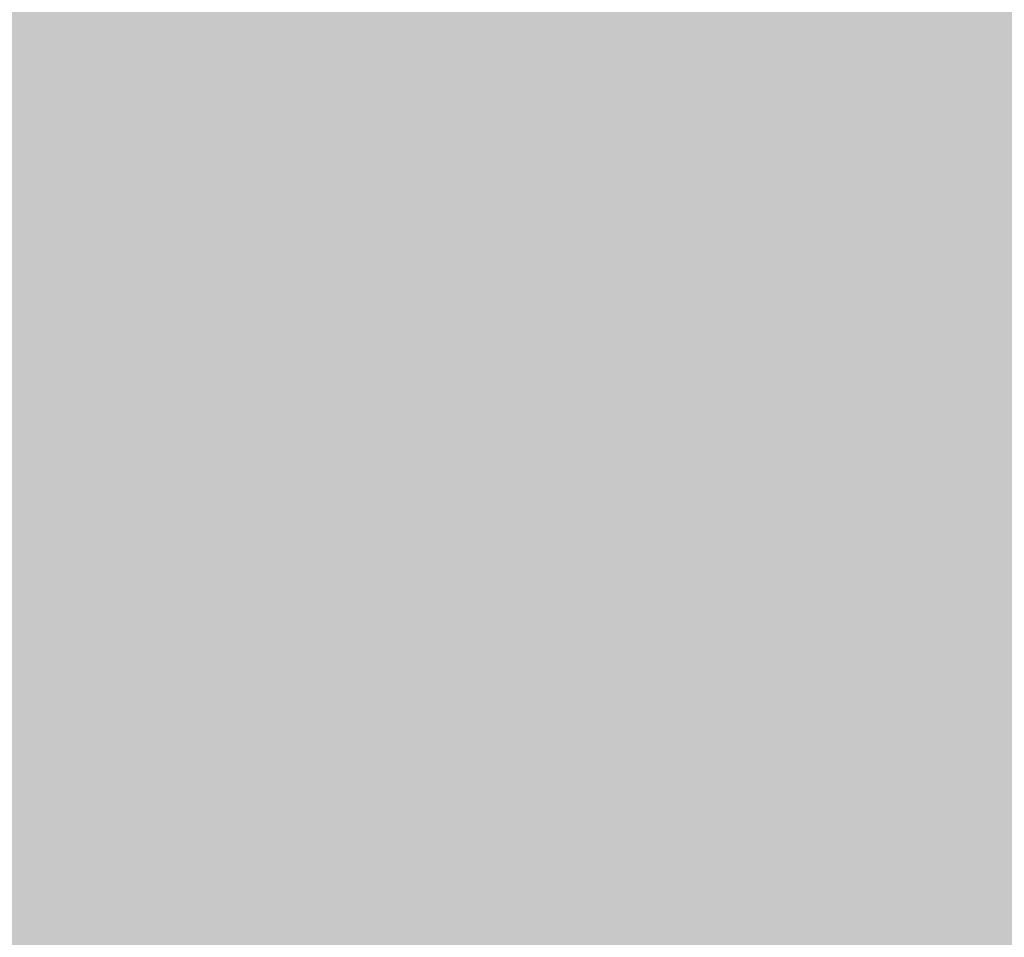
# Model space of a CAD drawing. Units: millimetres. Extents: x 0 to 2267, y 0 to 1823.
# Tile 143 of 256: x 1802 to 1823, y 1132 to 1152. Entities that reach past the tile are written whole.
import ezdxf

# ---------------------------------------------------------------- set-up
doc = ezdxf.new("R2010")
doc.units = ezdxf.units.MM
doc.header["$MEASUREMENT"] = 0
doc.layers.add('M-HATC', color=252, linetype='Continuous', lineweight=18)

msp = doc.modelspace()

# ---------------------------------------------------------------- hatches: boundary and pattern name
at = {"layer": 'M-HATC'}
h = msp.add_hatch(color=256, dxfattribs=at)
h.dxf.hatch_style = 1
h.paths.add_polyline_path([(2055.771, 1603.062), (1381.087, 1603.062), (1381.087, 1598.062), (2055.771, 1598.062)])
h.paths.add_polyline_path([(2055.771, 1598.062), (1381.087, 1598.062), (1381.087, 1593.062), (2055.771, 1593.062)])
h.paths.add_polyline_path([(2051.307, 1536.761), (1385.55, 1536.761), (1385.55, 1526.761), (1387.55, 1526.761), (1388.537, 1525.053), (1385.332, 1521.233), (1385.332, 1521.223), (2050.254, 1522.749), (2048.321, 1525.053), (2049.307, 1526.761), (2051.307, 1526.761)])
edge = h.paths.add_edge_path()
edge.add_arc((1847.535, 1379.149), 135, 222.60306, 222.89085, ccw=False)
edge.add_line((1748.166, 1287.766), (1683.092, 1287.766))
edge.add_arc((1583.724, 1379.149), 135, 317.10915, 317.39694, ccw=False)
edge.add_arc((1678.969, 1290.671), 5, 222.8909, 317.1091, ccw=False)
edge.add_arc((1774.213, 1379.149), 135, 222.60306, 222.89085, ccw=False)
edge.add_line((1674.845, 1287.766), (1609.771, 1287.766))
edge.add_arc((1510.403, 1379.149), 135, 317.10915, 317.39694, ccw=False)
edge.add_arc((1605.647, 1290.671), 5, 222.8909, 317.1091, ccw=False)
edge.add_arc((1700.892, 1379.149), 135, 222.60306, 222.89085, ccw=False)
edge.add_line((1601.524, 1287.766), (1536.45, 1287.766))
edge.add_arc((1437.081, 1379.149), 135, 317.10915, 317.39694, ccw=False)
edge.add_arc((1532.326, 1290.671), 5, 222.8909, 317.1091, ccw=False)
edge.add_arc((1627.571, 1379.149), 135, 222.60306, 222.89085, ccw=False)
edge.add_line((1528.203, 1287.766), (1505.929, 1287.766))
edge.add_spline(control_points=[(1505.929, 1287.766), (1504.262, 1287.766), (1504.262, 1282.766), (1505.929, 1282.766)], knot_values=[0, 0, 0, 0, 5, 5, 5, 5], degree=3, periodic=0)
edge.add_line((1505.929, 1282.766), (1930.929, 1282.766))
edge.add_spline(control_points=[(1930.929, 1282.766), (1932.596, 1282.766), (1932.596, 1287.766), (1930.929, 1287.766)], knot_values=[0, 0, 0, 0, 5, 5, 5, 5], degree=3, periodic=0)
edge.add_line((1930.929, 1287.766), (1903.056, 1287.766))
edge.add_arc((1803.688, 1379.149), 135, 317.10915, 317.39694, ccw=False)
edge.add_arc((1898.932, 1290.671), 5, 222.8909, 317.1091, ccw=False)
edge.add_arc((1994.177, 1379.149), 135, 222.60306, 222.89085, ccw=False)
edge.add_line((1894.809, 1287.766), (1829.735, 1287.766))
edge.add_arc((1730.366, 1379.149), 135, 317.10915, 317.39694, ccw=False)
edge.add_arc((1825.611, 1290.671), 5, 222.8909, 317.1091, ccw=False)
edge.add_arc((1920.856, 1379.149), 135, 222.60306, 222.89085, ccw=False)
edge.add_line((1821.487, 1287.766), (1756.413, 1287.766))
edge.add_arc((1657.045, 1379.149), 135, 317.10915, 317.39694, ccw=False)
edge.add_arc((1752.29, 1290.671), 5, 222.8909, 317.1091, ccw=False)
edge = h.paths.add_edge_path()
edge.add_spline(control_points=[(1843.429, 1227.247), (1845.096, 1227.247), (1845.096, 1232.247), (1843.429, 1232.247)], knot_values=[0, 0, 0, 0, 5, 5, 5, 5], degree=3, periodic=0)
edge.add_line((1843.429, 1232.247), (1593.429, 1232.247))
edge.add_spline(control_points=[(1593.429, 1232.247), (1591.762, 1232.247), (1591.762, 1227.247), (1593.429, 1227.247)], knot_values=[0, 0, 0, 0, 5, 5, 5, 5], degree=3, periodic=0)
edge.add_line((1593.429, 1227.247), (1843.429, 1227.247))
h.paths.add_polyline_path([(1905.929, 1127.417), (1530.929, 1127.417, 0.414214), (1520.929, 1117.417), (1530.929, 1117.417), (1915.929, 1117.417, 0.414214)])
edge = h.paths.add_edge_path()
edge.add_arc((1397.086, 1498.408), 12.73, 90.7821, 190.8787, ccw=False)
edge.add_line((1396.912, 1511.136), (1428.01, 1511.349))
edge.add_line((1428.01, 1511.349), (1433.01, 1511.349))
edge.add_line((1433.01, 1511.349), (1434.439, 1511.349))
edge.add_arc((1419.474, 1498.08), 20, 41.561, 74.0821)
edge.add_line((1424.959, 1517.314), (1399.935, 1517.256))
edge.add_spline(control_points=[(1399.931, 1517.256), (1399.884, 1517.213), (1399.833, 1517.169), (1399.777, 1517.124)], knot_values=[11.567499, 11.567499, 11.567499, 11.567499, 11.814249, 11.814249, 11.814249, 11.814249], degree=3, periodic=0)
edge.add_spline(control_points=[(1399.633, 1517.01), (1399.583, 1516.972), (1399.531, 1516.934), (1399.476, 1516.895)], knot_values=[11.167718, 11.167718, 11.167718, 11.167718, 11.365188, 11.365188, 11.365188, 11.365188], degree=3, periodic=0)
edge.add_spline(control_points=[(1399.34, 1516.8), (1399.151, 1516.672), (1398.938, 1516.538), (1398.704, 1516.399)], knot_values=[10.376405, 10.376405, 10.376405, 10.376405, 11.00994, 11.00994, 11.00994, 11.00994], degree=3, periodic=0)
edge.add_spline(control_points=[(1398.657, 1516.372), (1398.579, 1516.326), (1398.498, 1516.28), (1398.415, 1516.233)], knot_values=[10.125175, 10.125175, 10.125175, 10.125175, 10.334406, 10.334406, 10.334406, 10.334406], degree=3, periodic=0)
edge.add_spline(control_points=[(1398.264, 1516.149), (1398.196, 1516.111), (1398.126, 1516.073), (1398.055, 1516.035)], knot_values=[9.832246, 9.832246, 9.832246, 9.832246, 9.999658, 9.999658, 9.999658, 9.999658], degree=3, periodic=0)
edge.add_spline(control_points=[(1397.999, 1516.005), (1397.731, 1515.862), (1397.446, 1515.717), (1397.147, 1515.571)], knot_values=[9.161808, 9.161808, 9.161808, 9.161808, 9.787769, 9.787769, 9.787769, 9.787769], degree=3, periodic=0)
edge.add_spline(control_points=[(1397.147, 1515.571), (1396.842, 1515.423), (1396.522, 1515.274), (1396.191, 1515.126)], knot_values=[8.524455, 8.524455, 8.524455, 8.524455, 9.161808, 9.161808, 9.161808, 9.161808], degree=3, periodic=0)
edge.add_spline(control_points=[(1396.078, 1515.076), (1395.985, 1515.035), (1395.892, 1514.994), (1395.798, 1514.953)], knot_values=[8.275193, 8.275193, 8.275193, 8.275193, 8.451726, 8.451726, 8.451726, 8.451726], degree=3, periodic=0)
edge.add_spline(control_points=[(1395.602, 1514.869), (1395.5, 1514.826), (1395.397, 1514.782), (1395.293, 1514.739)], knot_values=[7.962917, 7.962917, 7.962917, 7.962917, 8.152764, 8.152764, 8.152764, 8.152764], degree=3, periodic=0)
edge.add_spline(control_points=[(1395.212, 1514.706), (1394.828, 1514.547), (1394.435, 1514.393), (1394.036, 1514.244)], knot_values=[7.21254, 7.21254, 7.21254, 7.21254, 7.913148, 7.913148, 7.913148, 7.913148], degree=3, periodic=0)
edge.add_spline(control_points=[(1394.036, 1514.244), (1393.708, 1514.121), (1393.375, 1514.003), (1393.043, 1513.889)], knot_values=[6.633733, 6.633733, 6.633733, 6.633733, 7.21254, 7.21254, 7.21254, 7.21254], degree=3, periodic=0)
edge.add_spline(control_points=[(1392.821, 1513.815), (1392.72, 1513.781), (1392.618, 1513.748), (1392.517, 1513.715)], knot_values=[6.328796, 6.328796, 6.328796, 6.328796, 6.505493, 6.505493, 6.505493, 6.505493], degree=3, periodic=0)
edge.add_spline(control_points=[(1392.517, 1513.715), (1392.319, 1513.652), (1392.121, 1513.59), (1391.924, 1513.531)], knot_values=[5.984605, 5.984605, 5.984605, 5.984605, 6.328796, 6.328796, 6.328796, 6.328796], degree=3, periodic=0)
edge.add_spline(control_points=[(1391.792, 1513.491), (1391.312, 1513.35), (1390.838, 1513.224), (1390.378, 1513.117)], knot_values=[5.066697, 5.066697, 5.066697, 5.066697, 5.907055, 5.907055, 5.907055, 5.907055], degree=3, periodic=0)
edge.add_spline(control_points=[(1390.378, 1513.117), (1390.18, 1513.071), (1389.984, 1513.028), (1389.791, 1512.99)], knot_values=[4.70367, 4.70367, 4.70367, 4.70367, 5.066695, 5.066695, 5.066695, 5.066695], degree=3, periodic=0)
edge.add_spline(control_points=[(1389.422, 1512.92), (1389.246, 1512.889), (1389.073, 1512.862), (1388.904, 1512.838)], knot_values=[4.130571, 4.130571, 4.130571, 4.130571, 4.469816, 4.469816, 4.469816, 4.469816], degree=3, periodic=0)
edge.add_spline(control_points=[(1388.904, 1512.838), (1388.591, 1512.795), (1388.291, 1512.764), (1388.007, 1512.749)], knot_values=[3.504031, 3.504031, 3.504031, 3.504031, 4.130571, 4.130571, 4.130571, 4.130571], degree=3, periodic=0)
edge.add_spline(control_points=[(1387.936, 1512.746), (1387.854, 1512.742), (1387.773, 1512.74), (1387.694, 1512.739)], knot_values=[3.268866, 3.268866, 3.268866, 3.268866, 3.451164, 3.451164, 3.451164, 3.451164], degree=3, periodic=0)
edge.add_spline(control_points=[(1387.335, 1512.744), (1387.208, 1512.75), (1387.085, 1512.76), (1386.967, 1512.774)], knot_values=[2.670686, 2.670686, 2.670686, 2.670686, 2.984, 2.984, 2.984, 2.984], degree=3, periodic=0)
edge.add_spline(control_points=[(1386.833, 1512.792), (1386.821, 1512.794), (1386.809, 1512.796), (1386.797, 1512.798)], knot_values=[2.516981, 2.516981, 2.516981, 2.516981, 2.549528, 2.549528, 2.549528, 2.549528], degree=3, periodic=0)
edge.add_spline(control_points=[(1386.453, 1512.873), (1386.426, 1512.881), (1386.399, 1512.889), (1386.373, 1512.897)], knot_values=[2.095869, 2.095869, 2.095869, 2.095869, 2.17941, 2.17941, 2.17941, 2.17941], degree=3, periodic=0)
edge.add_spline(control_points=[(1386.069, 1513.019), (1386.063, 1513.022), (1386.058, 1513.025), (1386.052, 1513.028)], knot_values=[1.72453, 1.72453, 1.72453, 1.72453, 1.745933, 1.745933, 1.745933, 1.745933], degree=3, periodic=0)
edge.add_arc((1399.474, 1498.08), 20, 131.8243, 180)
edge.add_arc((1630.334, 1505.548), 250.971, 181.70518, 236.42798)
edge.add_arc((1605.34, 1483.304), 218.782, 238.66083, 243.34961)
edge.add_arc((1647.091, 1510.359), 262.899, 183.12984, 237.85344, ccw=False)
h.paths.add_polyline_path([(1406.537, 1391.964, 0.149382), (1491.551, 1296.442, -0.129517)], flags=17)
edge = h.paths.add_edge_path()
edge.add_arc((2037.384, 1498.08), 20, 0, 48.2659)
edge.add_spline(control_points=[(2050.697, 1513.005), (2050.651, 1512.985), (2050.603, 1512.966), (2050.554, 1512.948)], knot_values=[1.835652, 1.835652, 1.835652, 1.835652, 2.000781, 2.000781, 2.000781, 2.000781], degree=3, periodic=0)
edge.add_spline(control_points=[(2050.462, 1512.917), (2050.479, 1512.922), (2050.496, 1512.928), (2050.513, 1512.934)], knot_values=[2.045477, 2.045477, 2.045477, 2.045477, 2.101389, 2.101389, 2.101389, 2.101389], degree=3, periodic=0)
edge.add_spline(control_points=[(2050.129, 1512.834), (2050.198, 1512.847), (2050.266, 1512.862), (2050.331, 1512.879)], knot_values=[2.237629, 2.237629, 2.237629, 2.237629, 2.435841, 2.435841, 2.435841, 2.435841], degree=3, periodic=0)
edge.add_spline(control_points=[(2050.095, 1512.828), (2050.106, 1512.83), (2050.118, 1512.832), (2050.129, 1512.834)], knot_values=[2.435841, 2.435841, 2.435841, 2.435841, 2.468321, 2.468321, 2.468321, 2.468321], degree=3, periodic=0)
edge.add_spline(control_points=[(2049.784, 1512.785), (2049.855, 1512.792), (2049.924, 1512.801), (2049.992, 1512.811)], knot_values=[2.563852, 2.563852, 2.563852, 2.563852, 2.748541, 2.748541, 2.748541, 2.748541], degree=3, periodic=0)
edge.add_spline(control_points=[(2049.405, 1512.762), (2049.536, 1512.765), (2049.663, 1512.773), (2049.784, 1512.785)], knot_values=[2.748541, 2.748541, 2.748541, 2.748541, 3.064882, 3.064882, 3.064882, 3.064882], degree=3, periodic=0)
edge.add_spline(control_points=[(2049.17, 1512.76), (2049.234, 1512.759), (2049.297, 1512.759), (2049.358, 1512.761)], knot_values=[3.102309, 3.102309, 3.102309, 3.102309, 3.2503, 3.2503, 3.2503, 3.2503], degree=3, periodic=0)
edge.add_spline(control_points=[(2048.857, 1512.769), (2048.964, 1512.764), (2049.068, 1512.761), (2049.17, 1512.76)], knot_values=[3.2503, 3.2503, 3.2503, 3.2503, 3.486069, 3.486069, 3.486069, 3.486069], degree=3, periodic=0)
edge.add_spline(control_points=[(2048.692, 1512.779), (2048.373, 1512.801), (2048.035, 1512.841), (2047.682, 1512.897)], knot_values=[3.606429, 3.606429, 3.606429, 3.606429, 4.2989, 4.2989, 4.2989, 4.2989], degree=3, periodic=0)
edge.add_spline(control_points=[(2047.682, 1512.897), (2047.546, 1512.919), (2047.408, 1512.942), (2047.268, 1512.969)], knot_values=[4.2989, 4.2989, 4.2989, 4.2989, 4.565769, 4.565769, 4.565769, 4.565769], degree=3, periodic=0)
edge.add_spline(control_points=[(2047.268, 1512.969), (2047.145, 1512.991), (2047.021, 1513.016), (2046.895, 1513.042)], knot_values=[4.565769, 4.565769, 4.565769, 4.565769, 4.799971, 4.799971, 4.799971, 4.799971], degree=3, periodic=0)
edge.add_spline(control_points=[(2046.895, 1513.042), (2046.529, 1513.119), (2046.151, 1513.209), (2045.768, 1513.311)], knot_values=[4.799971, 4.799971, 4.799971, 4.799971, 5.483718, 5.483718, 5.483718, 5.483718], degree=3, periodic=0)
edge.add_spline(control_points=[(2045.768, 1513.311), (2045.372, 1513.415), (2044.97, 1513.532), (2044.566, 1513.659)], knot_values=[5.483718, 5.483718, 5.483718, 5.483718, 6.187866, 6.187866, 6.187866, 6.187866], degree=3, periodic=0)
edge.add_spline(control_points=[(2044.566, 1513.659), (2044.415, 1513.706), (2044.263, 1513.755), (2044.112, 1513.805)], knot_values=[6.187866, 6.187866, 6.187866, 6.187866, 6.451551, 6.451551, 6.451551, 6.451551], degree=3, periodic=0)
edge.add_spline(control_points=[(2044.112, 1513.805), (2043.997, 1513.843), (2043.882, 1513.881), (2043.767, 1513.92)], knot_values=[6.451551, 6.451551, 6.451551, 6.451551, 6.651434, 6.651434, 6.651434, 6.651434], degree=3, periodic=0)
edge.add_spline(control_points=[(2043.767, 1513.92), (2043.372, 1514.055), (2042.977, 1514.198), (2042.589, 1514.346)], knot_values=[6.651434, 6.651434, 6.651434, 6.651434, 7.338879, 7.338879, 7.338879, 7.338879], degree=3, periodic=0)
edge.add_spline(control_points=[(2042.589, 1514.346), (2042.164, 1514.507), (2041.746, 1514.675), (2041.341, 1514.846)], knot_values=[7.338879, 7.338879, 7.338879, 7.338879, 8.089209, 8.089209, 8.089209, 8.089209], degree=3, periodic=0)
edge.add_spline(control_points=[(2041.341, 1514.846), (2041.103, 1514.946), (2040.869, 1515.048), (2040.64, 1515.15)], knot_values=[8.089209, 8.089209, 8.089209, 8.089209, 8.529587, 8.529587, 8.529587, 8.529587], degree=3, periodic=0)
edge.add_spline(control_points=[(2040.51, 1515.209), (2040.082, 1515.402), (2039.675, 1515.597), (2039.295, 1515.789)], knot_values=[8.613818, 8.613818, 8.613818, 8.613818, 9.44571, 9.44571, 9.44571, 9.44571], degree=3, periodic=0)
edge.add_spline(control_points=[(2039.295, 1515.789), (2039.062, 1515.907), (2038.839, 1516.025), (2038.629, 1516.14)], knot_values=[9.44571, 9.44571, 9.44571, 9.44571, 9.956404, 9.956404, 9.956404, 9.956404], degree=3, periodic=0)
edge.add_spline(control_points=[(2038.629, 1516.14), (2038.519, 1516.2), (2038.412, 1516.26), (2038.309, 1516.319)], knot_values=[9.956404, 9.956404, 9.956404, 9.956404, 10.223542, 10.223542, 10.223542, 10.223542], degree=3, periodic=0)
edge.add_spline(control_points=[(2038.309, 1516.319), (2038.214, 1516.374), (2038.122, 1516.428), (2038.033, 1516.481)], knot_values=[10.223542, 10.223542, 10.223542, 10.223542, 10.47051, 10.47051, 10.47051, 10.47051], degree=3, periodic=0)
edge.add_spline(control_points=[(2038.033, 1516.481), (2037.786, 1516.63), (2037.564, 1516.773), (2037.372, 1516.909)], knot_values=[10.47051, 10.47051, 10.47051, 10.47051, 11.15767, 11.15767, 11.15767, 11.15767], degree=3, periodic=0)
edge.add_spline(control_points=[(2037.372, 1516.909), (2037.279, 1516.975), (2037.193, 1517.04), (2037.114, 1517.102)], knot_values=[11.15767, 11.15767, 11.15767, 11.15767, 11.49227, 11.49227, 11.49227, 11.49227], degree=3, periodic=0)
edge.add_spline(control_points=[(2036.856, 1517.326), (2036.915, 1517.269), (2036.981, 1517.21), (2037.056, 1517.149)], knot_values=[11.577341, 11.577341, 11.577341, 11.577341, 11.91035, 11.91035, 11.91035, 11.91035], degree=3, periodic=0)
edge.add_spline(control_points=[(2036.807, 1517.375), (2036.823, 1517.359), (2036.839, 1517.342), (2036.856, 1517.326)], knot_values=[11.91035, 11.91035, 11.91035, 11.91035, 12.007402, 12.007402, 12.007402, 12.007402], degree=3, periodic=0)
edge.add_spline(control_points=[(2036.702, 1517.494), (2036.71, 1517.483), (2036.72, 1517.472), (2036.729, 1517.461)], knot_values=[12.184155, 12.184155, 12.184155, 12.184155, 12.255409, 12.255409, 12.255409, 12.255409], degree=3, periodic=0)
edge.add_spline(control_points=[(2036.616, 1517.621), (2036.62, 1517.613), (2036.624, 1517.606), (2036.629, 1517.598)], knot_values=[12.487913, 12.487913, 12.487913, 12.487913, 12.541035, 12.541035, 12.541035, 12.541035], degree=3, periodic=0)
edge.add_spline(control_points=[(2036.563, 1517.786), (2036.564, 1517.779), (2036.564, 1517.773), (2036.565, 1517.766)], knot_values=[12.911761, 12.911761, 12.911761, 12.911761, 12.968286, 12.968286, 12.968286, 12.968286], degree=3, periodic=0)
edge.add_spline(control_points=[(2036.617, 1517.93), (2036.612, 1517.926), (2036.609, 1517.921), (2036.605, 1517.916)], knot_values=[13.382527, 13.382527, 13.382527, 13.382527, 13.433791, 13.433791, 13.433791, 13.433791], degree=3, periodic=0)
edge.add_spline(control_points=[(2036.749, 1518.017), (2036.736, 1518.012), (2036.724, 1518.006), (2036.712, 1518)], knot_values=[13.726299, 13.726299, 13.726299, 13.726299, 13.809928, 13.809928, 13.809928, 13.809928], degree=3, periodic=0)
edge.add_spline(control_points=[(2036.86, 1518.053), (2036.839, 1518.047), (2036.818, 1518.042), (2036.799, 1518.035)], knot_values=[13.910887, 13.910887, 13.910887, 13.910887, 14.02153, 14.02153, 14.02153, 14.02153], degree=3, periodic=0)
edge.add_line((2036.964, 1518.08), (2032.384, 1518.08))
edge.add_line((2032.384, 1518.08), (2027.384, 1518.08))
edge.add_line((2027.384, 1518.08), (2022.384, 1518.08))
edge.add_line((2022.384, 1518.08), (2017.384, 1518.08))
edge.add_arc((2017.384, 1498.08), 20, 90, 138.439)
edge.add_line((2002.419, 1511.349), (2003.848, 1511.349))
edge.add_line((2003.848, 1511.349), (2008.848, 1511.349))
edge.add_line((2008.848, 1511.349), (2039.772, 1511.138))
edge.add_arc((2039.772, 1498.408), 12.73, -10.8787, 90, ccw=False)
edge.add_arc((1789.767, 1510.359), 262.899, 302.14656, 356.87016, ccw=False)
edge.add_arc((1831.518, 1483.304), 218.782, 296.65039, 301.33917)
edge.add_arc((1806.524, 1505.548), 250.971, 303.57202, 358.29482)
h.paths.add_polyline_path([(2030.321, 1391.964, -0.129517), (1945.307, 1296.442, 0.149382)], flags=17)
edge = h.paths.add_edge_path()
edge.add_spline(control_points=[(2037.246, 1518.082), (2037.29, 1518.081), (2037.336, 1518.08), (2037.384, 1518.08)], knot_values=[0.000012, 0.000012, 0.000012, 0.000012, 0.144754, 0.144754, 0.144754, 0.144754], degree=3, periodic=0)
edge.add_line((2037.336, 1518.08), (2037.01, 1518.08))
edge.add_spline(control_points=[(2037.01, 1518.08), (2036.982, 1518.077), (2036.956, 1518.073), (2036.931, 1518.068)], knot_values=[14.13465, 14.13465, 14.13465, 14.13465, 14.247197, 14.247197, 14.247197, 14.247197], degree=3, periodic=0)
edge.add_spline(control_points=[(2036.931, 1518.068), (2036.928, 1518.067), (2036.924, 1518.067), (2036.921, 1518.066)], knot_values=[14.118315, 14.118315, 14.118315, 14.118315, 14.13465, 14.13465, 14.13465, 14.13465], degree=3, periodic=0)
edge.add_spline(control_points=[(2036.921, 1518.066), (2036.912, 1518.064), (2036.903, 1518.063), (2036.895, 1518.061)], knot_values=[14.078086, 14.078086, 14.078086, 14.078086, 14.118315, 14.118315, 14.118315, 14.118315], degree=3, periodic=0)
edge.add_spline(control_points=[(2036.895, 1518.061), (2036.883, 1518.058), (2036.872, 1518.056), (2036.86, 1518.053)], knot_values=[14.02153, 14.02153, 14.02153, 14.02153, 14.078086, 14.078086, 14.078086, 14.078086], degree=3, periodic=0)
edge.add_spline(control_points=[(2036.86, 1518.053), (2036.839, 1518.047), (2036.818, 1518.042), (2036.799, 1518.035)], knot_values=[13.910887, 13.910887, 13.910887, 13.910887, 14.02153, 14.02153, 14.02153, 14.02153], degree=3, periodic=0)
edge.add_spline(control_points=[(2036.799, 1518.035), (2036.798, 1518.035), (2036.797, 1518.035), (2036.797, 1518.035)], knot_values=[13.906906, 13.906906, 13.906906, 13.906906, 13.910887, 13.910887, 13.910887, 13.910887], degree=3, periodic=0)
edge.add_spline(control_points=[(2036.797, 1518.035), (2036.788, 1518.032), (2036.78, 1518.029), (2036.772, 1518.026)], knot_values=[13.857826, 13.857826, 13.857826, 13.857826, 13.906906, 13.906906, 13.906906, 13.906906], degree=3, periodic=0)
edge.add_spline(control_points=[(2036.772, 1518.026), (2036.764, 1518.023), (2036.756, 1518.02), (2036.749, 1518.017)], knot_values=[13.809928, 13.809928, 13.809928, 13.809928, 13.857826, 13.857826, 13.857826, 13.857826], degree=3, periodic=0)
edge.add_spline(control_points=[(2036.749, 1518.017), (2036.736, 1518.012), (2036.724, 1518.006), (2036.712, 1518)], knot_values=[13.726299, 13.726299, 13.726299, 13.726299, 13.809928, 13.809928, 13.809928, 13.809928], degree=3, periodic=0)
edge.add_spline(control_points=[(2036.712, 1518), (2036.712, 1518), (2036.712, 1518), (2036.711, 1518)], knot_values=[13.723993, 13.723993, 13.723993, 13.723993, 13.726299, 13.726299, 13.726299, 13.726299], degree=3, periodic=0)
edge.add_spline(control_points=[(2036.711, 1518), (2036.706, 1517.997), (2036.701, 1517.994), (2036.696, 1517.992)], knot_values=[13.686536, 13.686536, 13.686536, 13.686536, 13.723993, 13.723993, 13.723993, 13.723993], degree=3, periodic=0)
edge.add_spline(control_points=[(2036.696, 1517.992), (2036.692, 1517.989), (2036.687, 1517.987), (2036.683, 1517.984)], knot_values=[13.651251, 13.651251, 13.651251, 13.651251, 13.686536, 13.686536, 13.686536, 13.686536], degree=3, periodic=0)
edge.add_spline(control_points=[(2036.683, 1517.984), (2036.676, 1517.98), (2036.67, 1517.976), (2036.664, 1517.971)], knot_values=[13.596804, 13.596804, 13.596804, 13.596804, 13.651251, 13.651251, 13.651251, 13.651251], degree=3, periodic=0)
edge.add_spline(control_points=[(2036.664, 1517.971), (2036.664, 1517.971), (2036.663, 1517.971), (2036.663, 1517.971)], knot_values=[13.593956, 13.593956, 13.593956, 13.593956, 13.596804, 13.596804, 13.596804, 13.596804], degree=3, periodic=0)
edge.add_spline(control_points=[(2036.663, 1517.971), (2036.66, 1517.969), (2036.658, 1517.967), (2036.655, 1517.965)], knot_values=[13.570322, 13.570322, 13.570322, 13.570322, 13.593956, 13.593956, 13.593956, 13.593956], degree=3, periodic=0)
edge.add_spline(control_points=[(2036.655, 1517.965), (2036.653, 1517.963), (2036.65, 1517.961), (2036.647, 1517.959)], knot_values=[13.545477, 13.545477, 13.545477, 13.545477, 13.570322, 13.570322, 13.570322, 13.570322], degree=3, periodic=0)
edge.add_spline(control_points=[(2036.647, 1517.959), (2036.647, 1517.959), (2036.647, 1517.959), (2036.647, 1517.959)], knot_values=[13.543931, 13.543931, 13.543931, 13.543931, 13.545477, 13.545477, 13.545477, 13.545477], degree=3, periodic=0)
edge.add_spline(control_points=[(2036.647, 1517.959), (2036.641, 1517.954), (2036.636, 1517.949), (2036.631, 1517.945)], knot_values=[13.488237, 13.488237, 13.488237, 13.488237, 13.543931, 13.543931, 13.543931, 13.543931], degree=3, periodic=0)
edge.add_spline(control_points=[(2036.631, 1517.945), (2036.628, 1517.942), (2036.626, 1517.94), (2036.623, 1517.937)], knot_values=[13.460307, 13.460307, 13.460307, 13.460307, 13.488237, 13.488237, 13.488237, 13.488237], degree=3, periodic=0)
edge.add_spline(control_points=[(2036.623, 1517.937), (2036.622, 1517.936), (2036.62, 1517.934), (2036.618, 1517.932)], knot_values=[13.439712, 13.439712, 13.439712, 13.439712, 13.460307, 13.460307, 13.460307, 13.460307], degree=3, periodic=0)
edge.add_spline(control_points=[(2036.618, 1517.932), (2036.618, 1517.931), (2036.617, 1517.931), (2036.617, 1517.93)], knot_values=[13.433791, 13.433791, 13.433791, 13.433791, 13.439712, 13.439712, 13.439712, 13.439712], degree=3, periodic=0)
edge.add_spline(control_points=[(2036.617, 1517.93), (2036.612, 1517.926), (2036.609, 1517.921), (2036.605, 1517.916)], knot_values=[13.382527, 13.382527, 13.382527, 13.382527, 13.433791, 13.433791, 13.433791, 13.433791], degree=3, periodic=0)
edge.add_spline(control_points=[(2036.605, 1517.916), (2036.603, 1517.913), (2036.6, 1517.91), (2036.598, 1517.907)], knot_values=[13.350017, 13.350017, 13.350017, 13.350017, 13.382527, 13.382527, 13.382527, 13.382527], degree=3, periodic=0)
edge.add_spline(control_points=[(2036.598, 1517.907), (2036.597, 1517.906), (2036.596, 1517.904), (2036.595, 1517.903)], knot_values=[13.333922, 13.333922, 13.333922, 13.333922, 13.350017, 13.350017, 13.350017, 13.350017], degree=3, periodic=0)
edge.add_spline(control_points=[(2036.595, 1517.903), (2036.595, 1517.902), (2036.594, 1517.901), (2036.593, 1517.9)], knot_values=[13.323828, 13.323828, 13.323828, 13.323828, 13.333922, 13.333922, 13.333922, 13.333922], degree=3, periodic=0)
edge.add_spline(control_points=[(2036.593, 1517.9), (2036.59, 1517.895), (2036.588, 1517.891), (2036.585, 1517.886)], knot_values=[13.277545, 13.277545, 13.277545, 13.277545, 13.323828, 13.323828, 13.323828, 13.323828], degree=3, periodic=0)
edge.add_spline(control_points=[(2036.585, 1517.886), (2036.584, 1517.883), (2036.582, 1517.879), (2036.58, 1517.875)], knot_values=[13.240119, 13.240119, 13.240119, 13.240119, 13.277545, 13.277545, 13.277545, 13.277545], degree=3, periodic=0)
edge.add_spline(control_points=[(2036.58, 1517.875), (2036.58, 1517.874), (2036.579, 1517.873), (2036.578, 1517.872)], knot_values=[13.228211, 13.228211, 13.228211, 13.228211, 13.240119, 13.240119, 13.240119, 13.240119], degree=3, periodic=0)
edge.add_spline(control_points=[(2036.578, 1517.872), (2036.578, 1517.87), (2036.577, 1517.869), (2036.577, 1517.868)], knot_values=[13.215717, 13.215717, 13.215717, 13.215717, 13.228211, 13.228211, 13.228211, 13.228211], degree=3, periodic=0)
edge.add_spline(control_points=[(2036.577, 1517.868), (2036.575, 1517.864), (2036.574, 1517.86), (2036.573, 1517.857)], knot_values=[13.179847, 13.179847, 13.179847, 13.179847, 13.215717, 13.215717, 13.215717, 13.215717], degree=3, periodic=0)
edge.add_spline(control_points=[(2036.573, 1517.857), (2036.571, 1517.851), (2036.57, 1517.846), (2036.569, 1517.841)], knot_values=[13.132017, 13.132017, 13.132017, 13.132017, 13.179847, 13.179847, 13.179847, 13.179847], degree=3, periodic=0)
edge.add_spline(control_points=[(2036.569, 1517.841), (2036.568, 1517.84), (2036.568, 1517.839), (2036.568, 1517.838)], knot_values=[13.122482, 13.122482, 13.122482, 13.122482, 13.132017, 13.132017, 13.132017, 13.132017], degree=3, periodic=0)
edge.add_spline(control_points=[(2036.568, 1517.838), (2036.568, 1517.836), (2036.567, 1517.835), (2036.567, 1517.833)], knot_values=[13.105592, 13.105592, 13.105592, 13.105592, 13.122482, 13.122482, 13.122482, 13.122482], degree=3, periodic=0)
edge.add_spline(control_points=[(2036.567, 1517.833), (2036.566, 1517.829), (2036.566, 1517.826), (2036.565, 1517.822)], knot_values=[13.074063, 13.074063, 13.074063, 13.074063, 13.105592, 13.105592, 13.105592, 13.105592], degree=3, periodic=0)
edge.add_spline(control_points=[(2036.565, 1517.822), (2036.565, 1517.822), (2036.565, 1517.822), (2036.565, 1517.822)], knot_values=[13.074043, 13.074043, 13.074043, 13.074043, 13.074063, 13.074063, 13.074063, 13.074063], degree=3, periodic=0)
edge.add_spline(control_points=[(2036.565, 1517.822), (2036.564, 1517.816), (2036.564, 1517.811), (2036.564, 1517.805)], knot_values=[13.021884, 13.021884, 13.021884, 13.021884, 13.074043, 13.074043, 13.074043, 13.074043], degree=3, periodic=0)
edge.add_spline(control_points=[(2036.564, 1517.805), (2036.564, 1517.804), (2036.564, 1517.803), (2036.564, 1517.803)], knot_values=[13.01674, 13.01674, 13.01674, 13.01674, 13.021884, 13.021884, 13.021884, 13.021884], degree=3, periodic=0)
edge.add_spline(control_points=[(2036.564, 1517.803), (2036.563, 1517.801), (2036.563, 1517.798), (2036.563, 1517.796)], knot_values=[12.996438, 12.996438, 12.996438, 12.996438, 13.01674, 13.01674, 13.01674, 13.01674], degree=3, periodic=0)
edge.add_spline(control_points=[(2036.563, 1517.796), (2036.563, 1517.793), (2036.563, 1517.789), (2036.563, 1517.786)], knot_values=[12.968286, 12.968286, 12.968286, 12.968286, 12.996438, 12.996438, 12.996438, 12.996438], degree=3, periodic=0)
edge.add_spline(control_points=[(2036.563, 1517.786), (2036.564, 1517.779), (2036.564, 1517.773), (2036.565, 1517.766)], knot_values=[12.911761, 12.911761, 12.911761, 12.911761, 12.968286, 12.968286, 12.968286, 12.968286], degree=3, periodic=0)
edge.add_spline(control_points=[(2036.565, 1517.766), (2036.565, 1517.766), (2036.565, 1517.766), (2036.565, 1517.766)], knot_values=[12.911017, 12.911017, 12.911017, 12.911017, 12.911761, 12.911761, 12.911761, 12.911761], degree=3, periodic=0)
edge.add_spline(control_points=[(2036.565, 1517.766), (2036.565, 1517.762), (2036.566, 1517.759), (2036.566, 1517.756)], knot_values=[12.88528, 12.88528, 12.88528, 12.88528, 12.911017, 12.911017, 12.911017, 12.911017], degree=3, periodic=0)
edge.add_spline(control_points=[(2036.566, 1517.756), (2036.567, 1517.753), (2036.567, 1517.751), (2036.568, 1517.748)], knot_values=[12.862519, 12.862519, 12.862519, 12.862519, 12.88528, 12.88528, 12.88528, 12.88528], degree=3, periodic=0)
edge.add_spline(control_points=[(2036.568, 1517.748), (2036.568, 1517.747), (2036.568, 1517.747), (2036.568, 1517.746)], knot_values=[12.858885, 12.858885, 12.858885, 12.858885, 12.862519, 12.862519, 12.862519, 12.862519], degree=3, periodic=0)
edge.add_spline(control_points=[(2036.568, 1517.746), (2036.569, 1517.74), (2036.571, 1517.733), (2036.572, 1517.726)], knot_values=[12.8053, 12.8053, 12.8053, 12.8053, 12.858885, 12.858885, 12.858885, 12.858885], degree=3, periodic=0)
edge.add_spline(control_points=[(2036.572, 1517.726), (2036.573, 1517.723), (2036.574, 1517.719), (2036.576, 1517.715)], knot_values=[12.775176, 12.775176, 12.775176, 12.775176, 12.8053, 12.8053, 12.8053, 12.8053], degree=3, periodic=0)
edge.add_spline(control_points=[(2036.576, 1517.715), (2036.576, 1517.713), (2036.577, 1517.71), (2036.578, 1517.708)], knot_values=[12.756759, 12.756759, 12.756759, 12.756759, 12.775176, 12.775176, 12.775176, 12.775176], degree=3, periodic=0)
edge.add_spline(control_points=[(2036.578, 1517.708), (2036.578, 1517.707), (2036.578, 1517.706), (2036.579, 1517.705)], knot_values=[12.748742, 12.748742, 12.748742, 12.748742, 12.756759, 12.756759, 12.756759, 12.756759], degree=3, periodic=0)
edge.add_spline(control_points=[(2036.579, 1517.705), (2036.581, 1517.698), (2036.583, 1517.692), (2036.586, 1517.685)], knot_values=[12.69959, 12.69959, 12.69959, 12.69959, 12.748742, 12.748742, 12.748742, 12.748742], degree=3, periodic=0)
edge.add_spline(control_points=[(2036.586, 1517.685), (2036.588, 1517.68), (2036.59, 1517.675), (2036.592, 1517.669)], knot_values=[12.659038, 12.659038, 12.659038, 12.659038, 12.69959, 12.69959, 12.69959, 12.69959], degree=3, periodic=0)
edge.add_spline(control_points=[(2036.592, 1517.669), (2036.594, 1517.665), (2036.596, 1517.66), (2036.598, 1517.656)], knot_values=[12.626806, 12.626806, 12.626806, 12.626806, 12.659038, 12.659038, 12.659038, 12.659038], degree=3, periodic=0)
edge.add_spline(control_points=[(2036.598, 1517.656), (2036.598, 1517.655), (2036.599, 1517.654), (2036.599, 1517.653)], knot_values=[12.619394, 12.619394, 12.619394, 12.619394, 12.626806, 12.626806, 12.626806, 12.626806], degree=3, periodic=0)
edge.add_spline(control_points=[(2036.599, 1517.653), (2036.604, 1517.642), (2036.61, 1517.632), (2036.616, 1517.621)], knot_values=[12.541039, 12.541039, 12.541039, 12.541039, 12.619394, 12.619394, 12.619394, 12.619394], degree=3, periodic=0)
edge.add_spline(control_points=[(2036.616, 1517.621), (2036.616, 1517.621), (2036.616, 1517.621), (2036.616, 1517.621)], knot_values=[12.541035, 12.541035, 12.541035, 12.541035, 12.541039, 12.541039, 12.541039, 12.541039], degree=3, periodic=0)
edge.add_spline(control_points=[(2036.616, 1517.621), (2036.62, 1517.613), (2036.624, 1517.606), (2036.629, 1517.598)], knot_values=[12.487913, 12.487913, 12.487913, 12.487913, 12.541035, 12.541035, 12.541035, 12.541035], degree=3, periodic=0)
edge.add_spline(control_points=[(2036.629, 1517.598), (2036.633, 1517.592), (2036.637, 1517.585), (2036.641, 1517.579)], knot_values=[12.443982, 12.443982, 12.443982, 12.443982, 12.487913, 12.487913, 12.487913, 12.487913], degree=3, periodic=0)
edge.add_spline(control_points=[(2036.641, 1517.579), (2036.641, 1517.578), (2036.642, 1517.576), (2036.643, 1517.575)], knot_values=[12.434996, 12.434996, 12.434996, 12.434996, 12.443982, 12.443982, 12.443982, 12.443982], degree=3, periodic=0)
edge.add_spline(control_points=[(2036.643, 1517.575), (2036.653, 1517.56), (2036.664, 1517.544), (2036.676, 1517.528)], knot_values=[12.329647, 12.329647, 12.329647, 12.329647, 12.434996, 12.434996, 12.434996, 12.434996], degree=3, periodic=0)
edge.add_spline(control_points=[(2036.676, 1517.528), (2036.684, 1517.517), (2036.693, 1517.505), (2036.702, 1517.494)], knot_values=[12.255409, 12.255409, 12.255409, 12.255409, 12.329647, 12.329647, 12.329647, 12.329647], degree=3, periodic=0)
edge.add_spline(control_points=[(2036.702, 1517.494), (2036.71, 1517.483), (2036.72, 1517.472), (2036.729, 1517.461)], knot_values=[12.184155, 12.184155, 12.184155, 12.184155, 12.255409, 12.255409, 12.255409, 12.255409], degree=3, periodic=0)
edge.add_spline(control_points=[(2036.729, 1517.461), (2036.744, 1517.444), (2036.759, 1517.426), (2036.775, 1517.409)], knot_values=[12.075961, 12.075961, 12.075961, 12.075961, 12.184155, 12.184155, 12.184155, 12.184155], degree=3, periodic=0)
edge.add_spline(control_points=[(2036.775, 1517.409), (2036.776, 1517.407), (2036.777, 1517.406), (2036.778, 1517.405)], knot_values=[12.069502, 12.069502, 12.069502, 12.069502, 12.075961, 12.075961, 12.075961, 12.075961], degree=3, periodic=0)
edge.add_spline(control_points=[(2036.778, 1517.405), (2036.788, 1517.395), (2036.797, 1517.385), (2036.807, 1517.375)], knot_values=[12.007402, 12.007402, 12.007402, 12.007402, 12.069502, 12.069502, 12.069502, 12.069502], degree=3, periodic=0)
edge.add_spline(control_points=[(2036.807, 1517.375), (2036.823, 1517.359), (2036.839, 1517.342), (2036.856, 1517.326)], knot_values=[11.91035, 11.91035, 11.91035, 11.91035, 12.007402, 12.007402, 12.007402, 12.007402], degree=3, periodic=0)
edge.add_spline(control_points=[(2036.856, 1517.326), (2036.915, 1517.269), (2036.981, 1517.21), (2037.056, 1517.149)], knot_values=[11.577341, 11.577341, 11.577341, 11.577341, 11.91035, 11.91035, 11.91035, 11.91035], degree=3, periodic=0)
edge.add_spline(control_points=[(2037.056, 1517.149), (2037.075, 1517.134), (2037.094, 1517.118), (2037.114, 1517.102)], knot_values=[11.49227, 11.49227, 11.49227, 11.49227, 11.577341, 11.577341, 11.577341, 11.577341], degree=3, periodic=0)
edge.add_spline(control_points=[(2037.114, 1517.102), (2037.193, 1517.04), (2037.279, 1516.975), (2037.372, 1516.909)], knot_values=[11.15767, 11.15767, 11.15767, 11.15767, 11.49227, 11.49227, 11.49227, 11.49227], degree=3, periodic=0)
edge.add_spline(control_points=[(2037.372, 1516.909), (2037.564, 1516.773), (2037.786, 1516.63), (2038.033, 1516.481)], knot_values=[10.47051, 10.47051, 10.47051, 10.47051, 11.15767, 11.15767, 11.15767, 11.15767], degree=3, periodic=0)
edge.add_spline(control_points=[(2038.033, 1516.481), (2038.122, 1516.428), (2038.214, 1516.374), (2038.309, 1516.319)], knot_values=[10.223542, 10.223542, 10.223542, 10.223542, 10.47051, 10.47051, 10.47051, 10.47051], degree=3, periodic=0)
edge.add_spline(control_points=[(2038.309, 1516.319), (2038.412, 1516.26), (2038.519, 1516.2), (2038.629, 1516.14)], knot_values=[9.956404, 9.956404, 9.956404, 9.956404, 10.223542, 10.223542, 10.223542, 10.223542], degree=3, periodic=0)
edge.add_spline(control_points=[(2038.629, 1516.14), (2038.839, 1516.025), (2039.062, 1515.907), (2039.295, 1515.789)], knot_values=[9.44571, 9.44571, 9.44571, 9.44571, 9.956404, 9.956404, 9.956404, 9.956404], degree=3, periodic=0)
edge.add_spline(control_points=[(2039.295, 1515.789), (2039.675, 1515.597), (2040.082, 1515.402), (2040.51, 1515.209)], knot_values=[8.613818, 8.613818, 8.613818, 8.613818, 9.44571, 9.44571, 9.44571, 9.44571], degree=3, periodic=0)
edge.add_spline(control_points=[(2040.51, 1515.209), (2040.553, 1515.189), (2040.597, 1515.17), (2040.64, 1515.15)], knot_values=[8.529587, 8.529587, 8.529587, 8.529587, 8.613818, 8.613818, 8.613818, 8.613818], degree=3, periodic=0)
edge.add_spline(control_points=[(2040.64, 1515.15), (2040.869, 1515.048), (2041.103, 1514.946), (2041.341, 1514.846)], knot_values=[8.089209, 8.089209, 8.089209, 8.089209, 8.529587, 8.529587, 8.529587, 8.529587], degree=3, periodic=0)
edge.add_spline(control_points=[(2041.341, 1514.846), (2041.746, 1514.675), (2042.164, 1514.507), (2042.589, 1514.346)], knot_values=[7.338879, 7.338879, 7.338879, 7.338879, 8.089209, 8.089209, 8.089209, 8.089209], degree=3, periodic=0)
edge.add_spline(control_points=[(2042.589, 1514.346), (2042.977, 1514.198), (2043.372, 1514.055), (2043.767, 1513.92)], knot_values=[6.651434, 6.651434, 6.651434, 6.651434, 7.338879, 7.338879, 7.338879, 7.338879], degree=3, periodic=0)
edge.add_spline(control_points=[(2043.767, 1513.92), (2043.882, 1513.881), (2043.997, 1513.843), (2044.112, 1513.805)], knot_values=[6.451551, 6.451551, 6.451551, 6.451551, 6.651434, 6.651434, 6.651434, 6.651434], degree=3, periodic=0)
edge.add_spline(control_points=[(2044.112, 1513.805), (2044.263, 1513.755), (2044.415, 1513.706), (2044.566, 1513.659)], knot_values=[6.187866, 6.187866, 6.187866, 6.187866, 6.451551, 6.451551, 6.451551, 6.451551], degree=3, periodic=0)
edge.add_spline(control_points=[(2044.566, 1513.659), (2044.97, 1513.532), (2045.372, 1513.415), (2045.768, 1513.311)], knot_values=[5.483718, 5.483718, 5.483718, 5.483718, 6.187866, 6.187866, 6.187866, 6.187866], degree=3, periodic=0)
edge.add_spline(control_points=[(2045.768, 1513.311), (2046.151, 1513.209), (2046.529, 1513.119), (2046.895, 1513.042)], knot_values=[4.799971, 4.799971, 4.799971, 4.799971, 5.483718, 5.483718, 5.483718, 5.483718], degree=3, periodic=0)
edge.add_spline(control_points=[(2046.895, 1513.042), (2047.021, 1513.016), (2047.145, 1512.991), (2047.268, 1512.969)], knot_values=[4.565769, 4.565769, 4.565769, 4.565769, 4.799971, 4.799971, 4.799971, 4.799971], degree=3, periodic=0)
edge.add_spline(control_points=[(2047.268, 1512.969), (2047.408, 1512.942), (2047.546, 1512.919), (2047.682, 1512.897)], knot_values=[4.2989, 4.2989, 4.2989, 4.2989, 4.565769, 4.565769, 4.565769, 4.565769], degree=3, periodic=0)
edge.add_spline(control_points=[(2047.682, 1512.897), (2048.035, 1512.841), (2048.373, 1512.801), (2048.692, 1512.779)], knot_values=[3.606429, 3.606429, 3.606429, 3.606429, 4.2989, 4.2989, 4.2989, 4.2989], degree=3, periodic=0)
edge.add_spline(control_points=[(2048.692, 1512.779), (2048.748, 1512.775), (2048.803, 1512.772), (2048.857, 1512.769)], knot_values=[3.486069, 3.486069, 3.486069, 3.486069, 3.606429, 3.606429, 3.606429, 3.606429], degree=3, periodic=0)
edge.add_spline(control_points=[(2048.857, 1512.769), (2048.964, 1512.764), (2049.068, 1512.761), (2049.17, 1512.76)], knot_values=[3.2503, 3.2503, 3.2503, 3.2503, 3.486069, 3.486069, 3.486069, 3.486069], degree=3, periodic=0)
edge.add_spline(control_points=[(2049.17, 1512.76), (2049.234, 1512.759), (2049.297, 1512.759), (2049.358, 1512.761)], knot_values=[3.102309, 3.102309, 3.102309, 3.102309, 3.2503, 3.2503, 3.2503, 3.2503], degree=3, periodic=0)
edge.add_spline(control_points=[(2049.358, 1512.761), (2049.374, 1512.761), (2049.39, 1512.761), (2049.405, 1512.762)], knot_values=[3.064882, 3.064882, 3.064882, 3.064882, 3.102309, 3.102309, 3.102309, 3.102309], degree=3, periodic=0)
edge.add_spline(control_points=[(2049.405, 1512.762), (2049.536, 1512.765), (2049.663, 1512.773), (2049.784, 1512.785)], knot_values=[2.748541, 2.748541, 2.748541, 2.748541, 3.064882, 3.064882, 3.064882, 3.064882], degree=3, periodic=0)
edge.add_spline(control_points=[(2049.784, 1512.785), (2049.855, 1512.792), (2049.924, 1512.801), (2049.992, 1512.811)], knot_values=[2.563852, 2.563852, 2.563852, 2.563852, 2.748541, 2.748541, 2.748541, 2.748541], degree=3, periodic=0)
edge.add_spline(control_points=[(2049.992, 1512.811), (2050.026, 1512.816), (2050.061, 1512.822), (2050.095, 1512.828)], knot_values=[2.468321, 2.468321, 2.468321, 2.468321, 2.563852, 2.563852, 2.563852, 2.563852], degree=3, periodic=0)
edge.add_spline(control_points=[(2050.095, 1512.828), (2050.106, 1512.83), (2050.118, 1512.832), (2050.129, 1512.834)], knot_values=[2.435841, 2.435841, 2.435841, 2.435841, 2.468321, 2.468321, 2.468321, 2.468321], degree=3, periodic=0)
edge.add_spline(control_points=[(2050.129, 1512.834), (2050.198, 1512.847), (2050.266, 1512.862), (2050.331, 1512.879)], knot_values=[2.237629, 2.237629, 2.237629, 2.237629, 2.435841, 2.435841, 2.435841, 2.435841], degree=3, periodic=0)
edge.add_spline(control_points=[(2050.331, 1512.879), (2050.375, 1512.891), (2050.419, 1512.903), (2050.462, 1512.917)], knot_values=[2.101389, 2.101389, 2.101389, 2.101389, 2.237629, 2.237629, 2.237629, 2.237629], degree=3, periodic=0)
edge.add_spline(control_points=[(2050.462, 1512.917), (2050.479, 1512.922), (2050.496, 1512.928), (2050.513, 1512.934)], knot_values=[2.045477, 2.045477, 2.045477, 2.045477, 2.101389, 2.101389, 2.101389, 2.101389], degree=3, periodic=0)
edge.add_spline(control_points=[(2050.513, 1512.934), (2050.527, 1512.938), (2050.54, 1512.943), (2050.554, 1512.948)], knot_values=[2.000781, 2.000781, 2.000781, 2.000781, 2.045477, 2.045477, 2.045477, 2.045477], degree=3, periodic=0)
edge.add_spline(control_points=[(2050.554, 1512.948), (2050.603, 1512.966), (2050.651, 1512.985), (2050.697, 1513.005)], knot_values=[1.835652, 1.835652, 1.835652, 1.835652, 2.000781, 2.000781, 2.000781, 2.000781], degree=3, periodic=0)
edge.add_arc((2037.384, 1498.08), 20, 48.2659, 90.1299)
edge = h.paths.add_edge_path(flags=16)
edge.add_spline(control_points=[(1386.139, 1512.986), (1388.92, 1511.739), (1398.039, 1515.519), (1399.931, 1517.256)], knot_values=[1.831046, 1.831046, 1.831046, 1.831046, 11.814249, 11.814249, 11.814249, 11.814249], degree=3, periodic=0)
edge.add_line((1399.931, 1517.256), (1393.743, 1517.242))
edge.add_arc((1399.474, 1498.08), 20, 106.6501, 131.8173)
h = msp.add_hatch(color=256, dxfattribs=at)
h.dxf.hatch_style = 1
h.paths.add_polyline_path([(2042.889, 1580.18), (2055.771, 1593.062), (1381.087, 1593.062), (1393.969, 1580.18), (1374.086, 1560.296), (2062.772, 1560.296)])
h.paths.add_polyline_path([(1843.429, 1201.33), (1843.429, 1227.247), (1593.429, 1227.247), (1593.429, 1201.33, -0.228274), (1574.599, 1162.235), (1530.929, 1127.417), (1905.929, 1127.417), (1862.259, 1162.235, -0.228274)])

doc.saveas('drawing.dxf')
